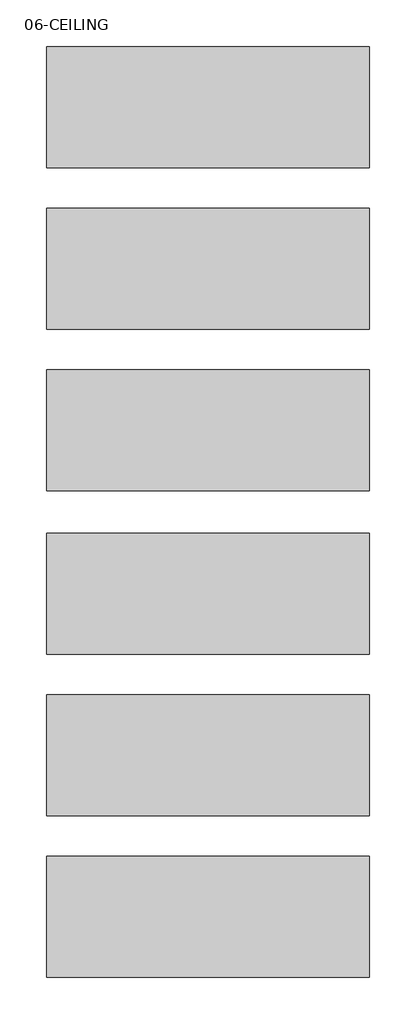
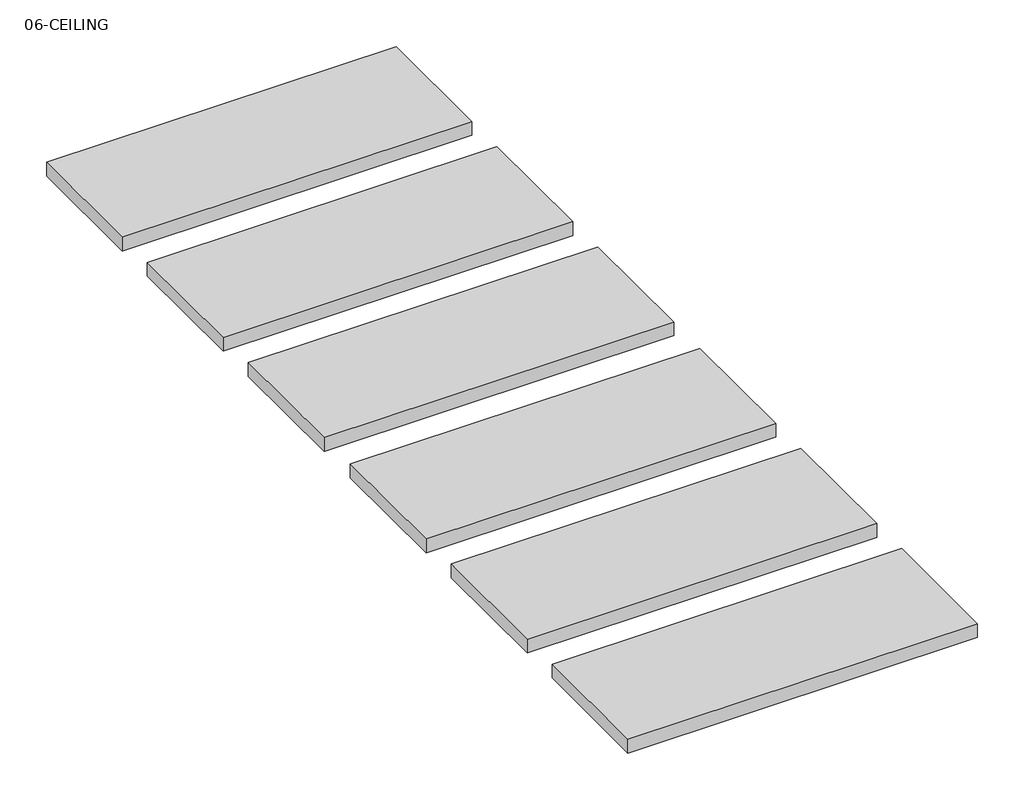
# One storey: 1 furniture element.
"""IFC4 building model written with IfcOpenShell, lengths in millimetres."""

from ifc_helpers import new_model, si_unit, origin, place, context, project, spatial, transform, mapped, element, save
from components import casework_1_casework_1_bf7433d0

model = new_model("IFC4")

# Units and contexts
model_context = context("Model", 3, world=origin())
ifc_project = project(units=[si_unit("LENGTHUNIT", "METRE", prefix="MILLI")], contexts=[model_context])

# Site, building, storey
site = spatial("IfcSite", under=ifc_project)
building = spatial("IfcBuilding", under=site)
storey = spatial("IfcBuildingStorey", under=building, Name="06-CEILING", Elevation=6750.0)

# Furniture
placement = place(None, origin())
casework_1_casework_1_shape = casework_1_casework_1_bf7433d0(model_context)
element("IfcFurniture", 1, ObjectType="Casework 1 : Casework 1", at=placement, inside=storey, context=model_context, shape_type="MappedRepresentation", body=[
    mapped(casework_1_casework_1_shape, transform((0.0, 0.0, 0.0), x_axis=(1.0, 0.0, 0.0), y_axis=(0.0, 1.0, 0.0), z_axis=(0.0, 0.0, 1.0))),
])

save(model, "model.ifc")

# Revit data of these elements
# Element 1 (IfcFurniture, "Casework 1 : Casework 1")
#   Phase Created = New Construction
#   Materials on its faces: "00-white plaster(1)"
# Materials
#   "00-white plaster(1)": class "Masonry", colour RGB 229 229 229, transparency 1, Description = "Common brick", Cost = 0
